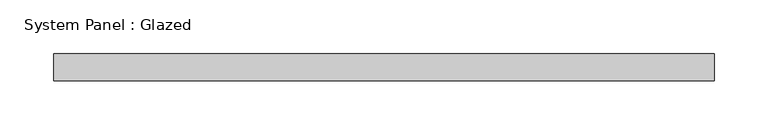
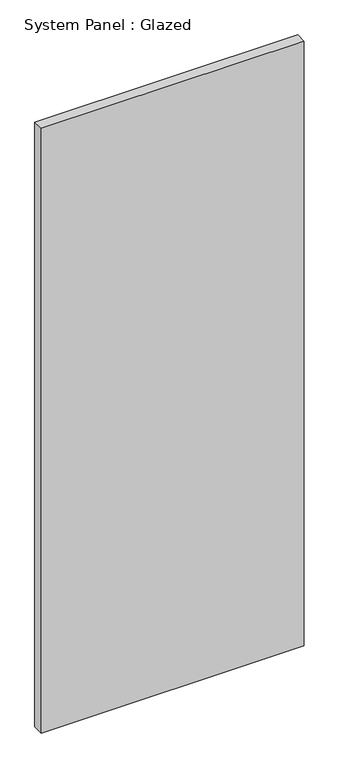
"""IFC4 building model written with IfcOpenShell, lengths in millimetres: plate geometry, System Panel : Glazed."""

from ifc_helpers import new_model, si_unit, origin, origin_with_axes, place, context, project, spatial, polyline, outline, extrude, source, transform, mapped, element, save


def system_panel_glazed_2c9823a4(model_context):
    return source(origin(), model_context, "Body", "SweptSolid", [
        extrude(outline(polyline([(307.975, 19.05), (-307.975, 19.05), (-307.975, 44.45), (307.975, 44.45), (307.975, 19.05)])), origin_with_axes(), (0.0, 0.0, 1.0), 1496.9353791),
    ])


if __name__ == "__main__":
    model = new_model("IFC4")
    model_context = context("Model", 3, world=origin())
    ifc_project = project(units=[si_unit("LENGTHUNIT", "METRE", prefix="MILLI")], contexts=[model_context])
    site = spatial("IfcSite", under=ifc_project)
    building = spatial("IfcBuilding", under=site)
    placement = place(None, origin())
    system_panel_glazed_shape = system_panel_glazed_2c9823a4(model_context)
    element("IfcPlate", 1, ObjectType="System Panel : Glazed", at=placement, inside=building, context=model_context, shape_type="MappedRepresentation", body=[
        mapped(system_panel_glazed_shape, transform((0.0, 0.0, 0.0), x_axis=(1.0, 0.0, 0.0), y_axis=(0.0, 1.0, 0.0), z_axis=(0.0, 0.0, 1.0))),
    ])
    save(model, "model.ifc")

# Revit data of these elements
# Type "System Panel : Glazed"
#   Construction Type Id = "GSP4R"
#   Analytic Construction = "1/8 in Pilkington single glazing"
#   Visual Light Transmittance = 0.9
#   Solar Heat Gain Coefficient = 0.86
#   Heat Transfer Coefficient (U) = 1.18115 BTU/(h·ft²·°F)
#   Define Thermal Properties by = 1
# Element 1 (IfcPlate, "System Panel : Glazed")
#   Materials on its faces: "Glass"
# Materials
#   "Glass": class "Glass", colour RGB 0 128 192, transparency 0.75, Description = "Soda Lime Glass", Cost = 0
